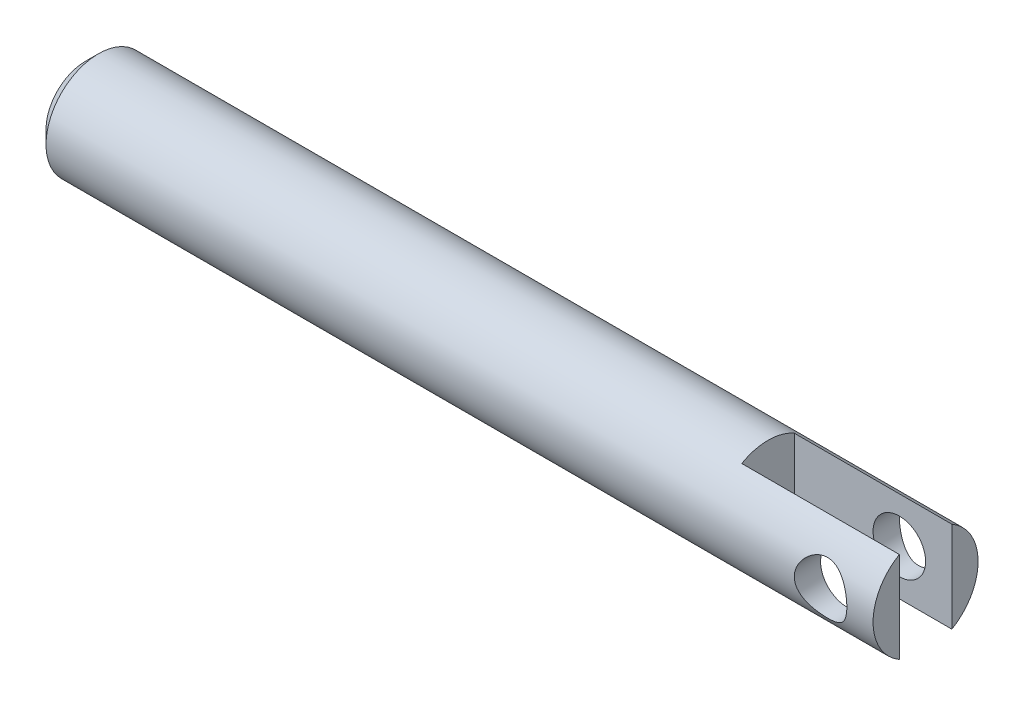
from build123d import *

# Parameters (mm, degrees)
ROD_PROFILE_SKETCH_W      = 4
ROD_PROFILE_SKETCH_H      = 0.25
END_NOTCH_SKETCH_R        = 0.125
END_NOTCH_CUT_DEPTH       = 5
CLEVIS_SLOT_SKETCH_W      = 0.75
CLEVIS_SLOT_SKETCH_H      = 0.25
CLEVIS_SLOT_DEPTH         = 5
CROSS_PIN_HOLE_SKETCH_R   = 0.15625
CROSS_PIN_HOLE_DEPTH      = 1.75
END_CHAMFER_SIZE          = 0.0625
SCALE_TO_FINAL_SIZE_SCALE = 25.4


with BuildPart() as part:
    # Rod Profile Sketch → Rod Body (revolve)
    with BuildSketch(Plane.XY, mode=Mode.PRIVATE) as rod_body_sk:
        with Locations((0, 0.125)):
            Rectangle(ROD_PROFILE_SKETCH_W, ROD_PROFILE_SKETCH_H)
    revolve(rod_body_sk.sketch.rotate(Axis((-2.293403827, 0, 0), (1, 0, 0)), 90), axis=Axis((-2.293403827, 0, 0), (1, 0, 0)))

    # End Notch Sketch → End Notch Cut (cut, symmetric)
    with BuildSketch(Plane.XY):
        with Locations((1.75, 0)):
            Circle(END_NOTCH_SKETCH_R)
    extrude(amount=END_NOTCH_CUT_DEPTH, both=True, mode=Mode.SUBTRACT)

    # Clevis Slot Sketch → Clevis Slot (cut, symmetric)
    with BuildSketch(Plane(origin=(0, 0, 0), x_dir=(1, 0, 0), z_dir=(0, 1, 0))):
        with Locations((1.625, 0)):
            Rectangle(CLEVIS_SLOT_SKETCH_W, CLEVIS_SLOT_SKETCH_H)
    extrude(amount=CLEVIS_SLOT_DEPTH, both=True, mode=Mode.SUBTRACT)

    # Cross Pin Hole Sketch → Cross Pin Hole (cut)
    with BuildSketch(Plane.ZY.offset(2)):
        Circle(CROSS_PIN_HOLE_SKETCH_R)
    extrude(amount=-CROSS_PIN_HOLE_DEPTH, mode=Mode.SUBTRACT)

    # End Chamfer
    end_chamfer_edges = [part.edges().sort_by_distance(p)[0] for p in [
        (-2, 0, -0.25),
    ]]
    chamfer(end_chamfer_edges, length=END_CHAMFER_SIZE)


with BuildPart() as part_1:
    # Scale to Final Size: scaled about (0, 0, 0)
    add(part.part.scale(SCALE_TO_FINAL_SIZE_SCALE))


solid = part_1.part
